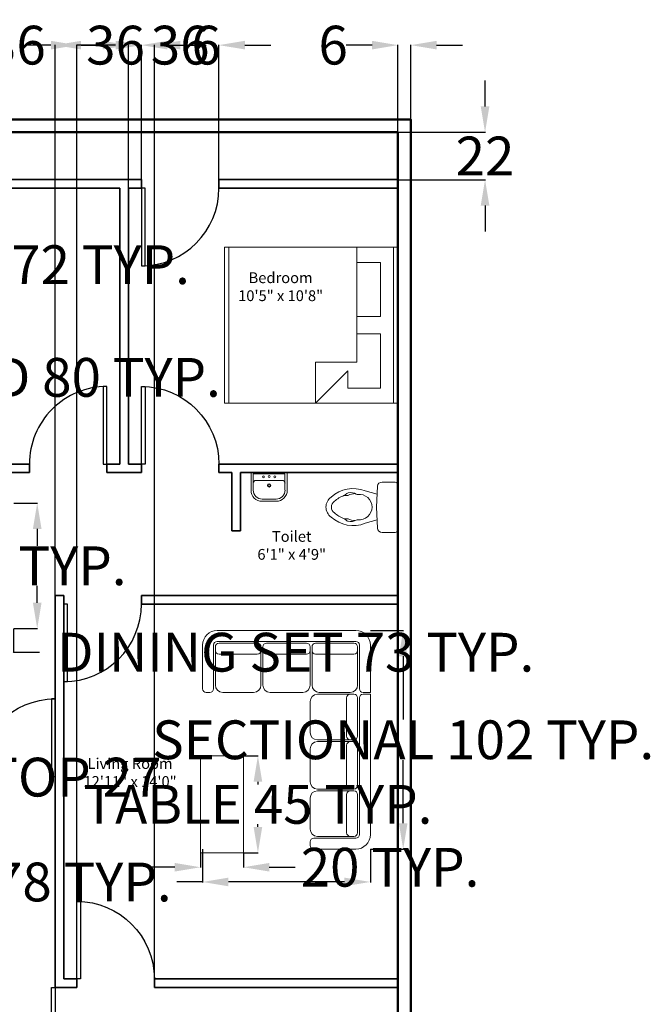
# Model space of a CAD drawing. Units: inches. Extents: x -230 to 384, y -962 to -183.
# Tile 6 of 6: x 91 to 384, y -640 to -183. Entities that reach past the tile are written whole.
import ezdxf

# ---------------------------------------------------------------- set-up
doc = ezdxf.new("R2010")
doc.units = ezdxf.units.IN
for name, color, linetype, lineweight in [('A-ANNO-DIMS', 2, 'Continuous', 18), ('A-AREA-IDEN', 7, 'Continuous', 18), ('A-DOOR', 3, 'Continuous', 25), ('A-FLOR-FIXT', 9, 'Continuous', 18), ('Furniture', 2, 'Continuous', 18), ('Inner Wall', 5, 'Continuous', 35), ('Outer Wall', 1, 'Continuous', 50)]:
    doc.layers.add(name, color=color, linetype=linetype, lineweight=lineweight)
doc.styles.get("Standard").update_dxf_attribs({"font": 'arial.ttf'})
doc.dimstyles.get("Standard").update_dxf_attribs({"dimtxt": 18, "dimasz": 12, "dimexe": 0.18, "dimexo": 0.0625, "dimgap": 0.09, "dimtad": 0, "dimtih": 1, "dimtoh": 1, "dimdec": 0, "dimzin": 0, "dimdsep": 46, "dimlunit": 3, "dimtxsty": 'Standard', "dimcen": 0.09, "dimadec": 0, "dimazin": 0, "dimtfac": 1, "dimtdec": 0, "dimtofl": 0, "dimtmove": 0, "dimatfit": 3, "dimfxl": 1, "dimtolj": 1, "dimtzin": 0, "dimarcsym": 0})

# ---------------------------------------------------------------- blocks, each defined once
blk = doc.blocks.new('*U2')
for p, q in [((0, 0), (0, 4)), ((36, 0), (36, 4))]:
    blk.add_line(p, q)
blk.add_lwpolyline([(0, 0), (0, -36), (1.75, -36), (1.75, 0)], close=True)
blk.add_arc((0, 0), 36, 270, 0)
blk = doc.blocks.new('*U4')
for p, q in [((0, 0), (0, -4)), ((36, 0), (36, -4))]:
    blk.add_line(p, q)
blk.add_lwpolyline([(0, 0), (0, 36), (1.75, 36), (1.75, 0)], close=True)
blk.add_arc((0, 0), 36, 0, 90)
blk = doc.blocks.new('A$C2AFA021D')
for p, q in [((0.8, 2.3), (0.2, 2.3)), ((0.85, 2.2), (0.85, 2.25)), ((0, 2.1), (0, 0.2)), ((0.15, 0.2), (0.15, 2.1)), ((0.175, 1.55), (0.175, 2.075)), ((0.2, 2.15), (0.8, 2.15)), ((0.225, 2.125), (0.275, 2.125)), ((0.75, 2.125), (0.275, 2.125)), ((0.325, 2.075), (0.325, 1.55)), ((0.85, 1.6), (0.85, 2.025)), ((0.275, 1.5), (0.225, 1.5)), ((0.275, 1.5), (0.75, 1.5)), ((0.175, 0.875), (0.175, 1.425)), ((0.225, 1.475), (0.275, 1.475)), ((0.75, 1.475), (0.275, 1.475)), ((0.325, 1.425), (0.325, 0.875)), ((0.85, 0.925), (0.85, 1.375)), ((0.275, 0.825), (0.225, 0.825)), ((0.275, 0.825), (0.75, 0.825)), ((0.975, 0.825), (1.4, 0.825)), ((1.625, 0.825), (2.075, 0.825)), ((2.3, 0.825), (2.725, 0.825)), ((2.9, 0.825), (2.95, 0.825)), ((0.175, 0.225), (0.175, 0.75)), ((0.225, 0.8), (0.275, 0.8)), ((0.75, 0.8), (0.275, 0.8)), ((0.325, 0.75), (0.325, 0.225)), ((0.85, 0.275), (0.85, 0.7)), ((0.875, 0.275), (0.875, 0.725)), ((1.5, 0.725), (1.5, 0.275)), ((1.525, 0.275), (1.525, 0.725)), ((2.175, 0.725), (2.175, 0.275)), ((2.2, 0.275), (2.2, 0.725)), ((2.825, 0.725), (2.825, 0.275)), ((2.85, 0.2), (2.85, 0.775)), ((3, 0.775), (3, 0.2)), ((0.875, 0.275), (0.875, 0.225)), ((1.45, 0.325), (0.925, 0.325)), ((1.5, 0.225), (1.5, 0.275)), ((1.525, 0.275), (1.525, 0.225)), ((2.125, 0.325), (1.575, 0.325)), ((2.175, 0.225), (2.175, 0.275)), ((2.2, 0.275), (2.2, 0.225)), ((2.775, 0.325), (2.25, 0.325)), ((2.825, 0.225), (2.825, 0.275)), ((0.8, 0.15), (0.2, 0.15)), ((0.275, 0.175), (0.225, 0.175)), ((0.275, 0.175), (0.75, 0.175)), ((0.925, 0.175), (1.45, 0.175)), ((0.925, 0.15), (2.8, 0.15)), ((1.575, 0.175), (2.125, 0.175)), ((2.25, 0.175), (2.775, 0.175)), ((0.85, 0), (0.85, 0.1)), ((0.875, 0.1), (0.875, 0)), ((0.2, 0), (0.85, 0)), ((2.8, 0), (0.875, 0))]:
    blk.add_line(p, q)
for centre, radius, start, end in [((0.2, 2.1), 0.2, 90, 180), ((0.8, 2.25), 0.05, 0, 90), ((0.8, 2.2), 0.05, 270, 0), ((0.2, 2.1), 0.05, 90, 180), ((0.225, 2.075), 0.05, 90, 180), ((0.275, 2.075), 0.05, 0, 90), ((0.75, 2.025), 0.1, 0, 90), ((0.225, 1.55), 0.05, 180, 270), ((0.275, 1.55), 0.05, 270, 0), ((0.75, 1.6), 0.1, 270, 0), ((0.225, 1.425), 0.05, 90, 180), ((0.275, 1.425), 0.05, 0, 90), ((0.75, 1.375), 0.1, 360, 90), ((0.225, 0.875), 0.05, 180, 270), ((0.275, 0.875), 0.05, 270, 0), ((0.75, 0.925), 0.1, 270, 0), ((0.975, 0.725), 0.1, 90, 180), ((1.4, 0.725), 0.1, 0, 90), ((1.625, 0.725), 0.1, 90, 180), ((2.075, 0.725), 0.1, 0, 90), ((2.3, 0.725), 0.1, 90, 180), ((2.725, 0.725), 0.1, 0, 90), ((2.9, 0.775), 0.05, 90, 180), ((2.95, 0.775), 0.05, 0, 90), ((0.225, 0.75), 0.05, 90, 180), ((0.275, 0.75), 0.05, 0, 90), ((0.75, 0.7), 0.1, 0, 90), ((0.75, 0.275), 0.1, 270, 0), ((0.925, 0.275), 0.05, 90, 180), ((1.45, 0.275), 0.05, 360, 90), ((1.575, 0.275), 0.05, 90, 180), ((2.125, 0.275), 0.05, 360, 90), ((2.25, 0.275), 0.05, 90, 180), ((2.775, 0.275), 0.05, 360, 90), ((0.2, 0.2), 0.2, 180, 270), ((0.2, 0.2), 0.05, 180, 270), ((0.225, 0.225), 0.05, 180, 270), ((0.275, 0.225), 0.05, 270, 0), ((0.8, 0.1), 0.05, 0, 90), ((0.925, 0.225), 0.05, 180, 270), ((0.925, 0.1), 0.05, 90, 180), ((1.45, 0.225), 0.05, 270, 0), ((1.575, 0.225), 0.05, 180, 270), ((2.125, 0.225), 0.05, 270, 0), ((2.25, 0.225), 0.05, 180, 270), ((2.775, 0.225), 0.05, 270, 0), ((2.8, 0.2), 0.2, 270, 0), ((2.8, 0.2), 0.05, 270, 0)]:
    blk.add_arc(centre, radius, start, end)
blk = doc.blocks.new('KING-00')
for p, q in [((-0.897, -0.947), (-0.897, 0.882)), ((0.602, 0.882), (0.602, -0.464)), ((1.034, -0.947), (1.034, 0.882)), ((0.602, 0.704), (0.881, 0.704)), ((0.881, 0.069), (0.881, 0.704)), ((0.602, 0.069), (0.881, 0.069)), ((0.881, -0.134), (0.602, -0.134)), ((0.881, -0.769), (0.881, -0.134)), ((0.119, -0.464), (0.119, -0.947)), ((0.602, -0.464), (0.119, -0.464)), ((0.119, -0.947), (0.5, -0.566)), ((0.5, -0.769), (0.5, -0.566)), ((0.5, -0.769), (0.881, -0.769))]:
    blk.add_line(p, q)
blk.add_lwpolyline([(-0.948, -0.947), (-0.948, 0.882), (1.084, 0.882), (1.084, -0.947)], close=True)
blk = doc.blocks.new('A$C1308471B')
at = {"ltscale": 20}
for p, q in [((0.0354, 0.4793), (0.1495, 0.4793)), ((0, 0.4607), (0, 0.0186)), ((0.2013, 0.2397), (0.1923, 0.4384)), ((0.1957, 0.3639), (0.3109, 0.3953)), ((0.5021, 0.3528), (0.4724, 0.3528)), ((0.4982, 0.3575), (0.4822, 0.3709)), ((0.2013, 0.2397), (0.1923, 0.0409)), ((0.1959, 0.1193), (0.3109, 0.0879)), ((0.5021, 0.1304), (0.4724, 0.1304)), ((0.4982, 0.1257), (0.4822, 0.1123)), ((0.0354, 0), (0.1495, 0))]:
    blk.add_line(p, q, dxfattribs=at)
for centre, radius, start, end in [((0.0354, 0.4328), 0.0465, 90, 136.52689), ((0.1495, 0.4365), 0.0429, 2.57554, 90), ((0.006, 0.4607), 0.006, 136.52689, 180), ((0.4248, 0.1104), 0.3068, 47.41345, 111.79241), ((0.4494, 0.2636), 0.1148, 79.39683, 118.57415), ((0.4658, 0.3513), 0.0255, 50, 79.39683), ((0.3654, 0.2416), 0.1206, 83.35226, 180), ((0.3823, 0.3868), 0.0255, 263.35226, 298.57415), ((0.405, 0.2159), 0.153, 63.50202, 90.45216), ((0.5146, 0.377), 0.0255, 230, 251.38812), ((0.5021, 0.3273), 0.0255, 70.3751, 90), ((0.4248, 0.1104), 0.2558, 46.61198, 70.3751), ((0.5654, 0.2416), 0.065, 0, 57.29738), ((0.5654, 0.2416), 0.116, 0, 54.71147), ((0.3654, 0.2416), 0.1206, 180, 276.64774), ((0.4248, 0.3728), 0.2558, 289.6249, 313.38802), ((0.5654, 0.2416), 0.065, 302.70262, 0), ((0.5654, 0.2416), 0.116, 305.28853, 0), ((0.4248, 0.3728), 0.3068, 248.20759, 312.58655), ((0.3823, 0.0964), 0.0255, 61.42585, 96.64774), ((0.4494, 0.2196), 0.1148, 241.42585, 280.60317), ((0.405, 0.2673), 0.153, 269.54784, 296.49798), ((0.4658, 0.1319), 0.0255, 280.60317, 310), ((0.5146, 0.1062), 0.0255, 108.61188, 130), ((0.5021, 0.1559), 0.0255, 270, 289.6249), ((0.006, 0.0186), 0.006, 180, 223.47311), ((0.0354, 0.0465), 0.0465, 223.47311, 270), ((0.1495, 0.0429), 0.0429, 270, 357.42446)]:
    blk.add_arc(centre, radius, start, end, dxfattribs=at)
blk = doc.blocks.new('A$C57EA129C')
for p, q in [((0, 0.443), (0, 0.178)), ((0.016, 0.459), (0.563, 0.459)), ((0.036, 0.432), (0.036, 0.29)), ((0.045, 0.441), (0.535, 0.441)), ((0.08, 0.334), (0.499, 0.334)), ((0.544, 0.432), (0.544, 0.29)), ((0.579, 0.443), (0.579, 0.178)), ((0.036, 0.29), (0.036, 0.178)), ((0.544, 0.29), (0.544, 0.178)), ((0.178, 0.036), (0.401, 0.036)), ((0.178, 0), (0.401, 0))]:
    blk.add_line(p, q)
for centre, radius in [((0.198, 0.392), 0.0143), ((0.29, 0.396), 0.0156), ((0.381, 0.392), 0.0143), ((0.29, 0.255), 0.0267), ((0.29, 0.255), 0.0178)]:
    blk.add_circle(centre, radius)
for centre, radius, start, end in [((0.016, 0.443), 0.016, 90, 180), ((0.045, 0.432), 0.00891, 90, 180), ((0.08, 0.29), 0.0445, 90, 180), ((0.499, 0.29), 0.0445, 0, 90), ((0.535, 0.432), 0.00891, 0, 90), ((0.563, 0.443), 0.016, 0, 90), ((0.178, 0.178), 0.178, 180, 270), ((0.178, 0.178), 0.143, 180, 270), ((0.401, 0.178), 0.178, 270, 0), ((0.401, 0.178), 0.143, 270, 0)]:
    blk.add_arc(centre, radius, start, end)
blk = doc.blocks.new('TABLE-COFFEE-RECT')
blk.add_lwpolyline([(0, 44.94), (19.86, 44.94), (19.86, 0), (0, 0)], close=True)
blk = doc.blocks.new('*D16')
at = {"layer": 'A-ANNO-DIMS', "color": 0, "lineweight": -2, "transparency": 16777216}
for p, q in [((72.67, -308.78), (84.86, -308.78)), ((84.68, -320.78), (84.68, -339.62)), ((84.68, -377.25), (84.68, -358.42)), ((72.67, -389.25), (84.86, -389.25))]:
    blk.add_line(p, q, dxfattribs=at)
at = {"layer": 'A-ANNO-DIMS', "color": 0, "transparency": 16777216}
for points in [[(82.68, -320.78), (86.68, -320.78), (84.68, -308.78)], [(82.68, -377.25), (86.68, -377.25), (84.68, -389.25)]]:
    blk.add_solid(points, dxfattribs=at)
at = {"layer": 'Defpoints', "color": 0, "transparency": 16777216}
for p in [(72.61, -308.78), (72.61, -389.25), (84.68, -389.25)]:
    blk.add_point(p, dxfattribs=at)
at = {"layer": 'A-ANNO-DIMS', "color": 0, "transparency": 16777216, "insert": (84.68, -349.02), "char_height": 18, "attachment_point": 5}
blk.add_mtext('\\A1;KING BED 80 TYP.', dxfattribs=at)
blk = doc.blocks.new('*D17')
at = {"layer": 'A-ANNO-DIMS', "color": 0, "lineweight": -2, "transparency": 16777216}
for p, q in [((0.19, -308.72), (0.19, -296.53)), ((12.19, -296.71), (60.61, -296.71)), ((72.61, -308.72), (72.61, -296.53)), ((72.61, -296.71), (84.61, -296.71))]:
    blk.add_line(p, q, dxfattribs=at)
at = {"layer": 'A-ANNO-DIMS', "color": 0, "transparency": 16777216}
for points in [[(12.19, -294.71), (12.19, -298.71), (0.19, -296.71)], [(60.61, -294.71), (60.61, -298.71), (72.61, -296.71)]]:
    blk.add_solid(points, dxfattribs=at)
at = {"layer": 'Defpoints', "color": 0, "transparency": 16777216}
for p in [(72.61, -296.71), (0.19, -308.78), (72.61, -308.78)]:
    blk.add_point(p, dxfattribs=at)
at = {"layer": 'A-ANNO-DIMS', "color": 0, "transparency": 16777216, "insert": (128.44, -296.71), "char_height": 18, "attachment_point": 5}
blk.add_mtext('\\A1;72 TYP.', dxfattribs=at)
blk = doc.blocks.new('*D22')
at = {"layer": 'A-ANNO-DIMS', "color": 0, "lineweight": -2, "transparency": 16777216}
for p, q in [((253.7, -466.5), (269.04, -466.5)), ((268.86, -478.5), (268.86, -507.86)), ((268.86, -556.02), (268.86, -526.67)), ((253.7, -568.02), (269.04, -568.02))]:
    blk.add_line(p, q, dxfattribs=at)
at = {"layer": 'A-ANNO-DIMS', "color": 0, "transparency": 16777216}
for points in [[(266.86, -478.5), (270.86, -478.5), (268.86, -466.5)], [(266.86, -556.02), (270.86, -556.02), (268.86, -568.02)]]:
    blk.add_solid(points, dxfattribs=at)
at = {"layer": 'Defpoints', "color": 0, "transparency": 16777216}
for p in [(253.63, -466.5), (253.63, -568.02), (268.86, -568.02)]:
    blk.add_point(p, dxfattribs=at)
at = {"layer": 'A-ANNO-DIMS', "color": 0, "transparency": 16777216, "insert": (268.86, -517.26), "char_height": 18, "attachment_point": 5}
blk.add_mtext('\\A1;SECTIONAL 102 TYP.', dxfattribs=at)
blk = doc.blocks.new('*D23')
at = {"layer": 'A-ANNO-DIMS', "color": 0, "lineweight": -2, "transparency": 16777216}
for p, q in [((175.8, -568.08), (175.8, -583.43)), ((253.63, -568.08), (253.63, -583.43)), ((175.8, -583.25), (163.8, -583.25)), ((241.63, -583.25), (187.8, -583.25))]:
    blk.add_line(p, q, dxfattribs=at)
at = {"layer": 'A-ANNO-DIMS', "color": 0, "transparency": 16777216}
for points in [[(187.8, -581.25), (187.8, -585.25), (175.8, -583.25)], [(241.63, -581.25), (241.63, -585.25), (253.63, -583.25)]]:
    blk.add_solid(points, dxfattribs=at)
at = {"layer": 'Defpoints', "color": 0, "transparency": 16777216}
for p in [(175.8, -568.02), (253.63, -568.02), (175.8, -583.25)]:
    blk.add_point(p, dxfattribs=at)
at = {"layer": 'A-ANNO-DIMS', "color": 0, "transparency": 16777216, "insert": (119.97, -583.25), "char_height": 18, "attachment_point": 5}
blk.add_mtext('\\A1;78 TYP.', dxfattribs=at)
blk = doc.blocks.new('*D24')
at = {"layer": 'A-ANNO-DIMS', "color": 0, "lineweight": -2, "transparency": 16777216}
for p, q in [((14.93, -465.69), (14.93, -476.78)), ((88.09, -465.69), (88.09, -476.78)), ((26.93, -476.6), (76.09, -476.6)), ((88.09, -476.6), (100.09, -476.6))]:
    blk.add_line(p, q, dxfattribs=at)
at = {"layer": 'A-ANNO-DIMS', "color": 0, "transparency": 16777216}
for points in [[(26.93, -474.6), (26.93, -478.6), (14.93, -476.6)], [(76.09, -474.6), (76.09, -478.6), (88.09, -476.6)]]:
    blk.add_solid(points, dxfattribs=at)
at = {"layer": 'Defpoints', "color": 0, "transparency": 16777216}
for p in [(14.93, -465.63), (88.09, -465.63), (88.09, -476.6)]:
    blk.add_point(p, dxfattribs=at)
at = {"layer": 'A-ANNO-DIMS', "color": 0, "transparency": 16777216, "insert": (218.98, -476.6), "char_height": 18, "attachment_point": 5}
blk.add_mtext('\\A1;DINING SET 73 TYP.', dxfattribs=at)
blk = doc.blocks.new('*D25')
at = {"layer": 'A-ANNO-DIMS', "color": 0, "lineweight": -2, "transparency": 16777216}
for p, q in [((88.15, -407.34), (99.24, -407.34)), ((99.06, -419.34), (99.06, -427.2)), ((99.06, -453.63), (99.06, -445.76)), ((88.15, -465.63), (99.24, -465.63))]:
    blk.add_line(p, q, dxfattribs=at)
at = {"layer": 'A-ANNO-DIMS', "color": 0, "transparency": 16777216}
for points in [[(97.06, -419.34), (101.06, -419.34), (99.06, -407.34)], [(97.06, -453.63), (101.06, -453.63), (99.06, -465.63)]]:
    blk.add_solid(points, dxfattribs=at)
at = {"layer": 'Defpoints', "color": 0, "transparency": 16777216}
for p in [(88.09, -407.34), (99.06, -407.34), (88.09, -465.63)]:
    blk.add_point(p, dxfattribs=at)
at = {"layer": 'A-ANNO-DIMS', "color": 0, "transparency": 16777216, "insert": (99.06, -436.48), "char_height": 18, "attachment_point": 5}
blk.add_mtext('\\A1;58 TYP.', dxfattribs=at)
blk = doc.blocks.new('*D26')
at = {"layer": 'A-ANNO-DIMS', "color": 0, "lineweight": -2, "transparency": 16777216}
for p, q in [((194.78, -524.74), (201.64, -524.74)), ((201.46, -536.74), (201.46, -537.96)), ((201.46, -557.68), (201.46, -556.45)), ((194.78, -569.68), (201.64, -569.68))]:
    blk.add_line(p, q, dxfattribs=at)
at = {"layer": 'A-ANNO-DIMS', "color": 0, "transparency": 16777216}
for points in [[(199.46, -536.74), (203.46, -536.74), (201.46, -524.74)], [(199.46, -557.68), (203.46, -557.68), (201.46, -569.68)]]:
    blk.add_solid(points, dxfattribs=at)
at = {"layer": 'Defpoints', "color": 0, "transparency": 16777216}
for p in [(194.72, -524.74), (201.46, -524.74), (194.72, -569.68)]:
    blk.add_point(p, dxfattribs=at)
at = {"layer": 'A-ANNO-DIMS', "color": 0, "transparency": 16777216, "insert": (201.46, -547.21), "char_height": 18, "attachment_point": 5}
blk.add_mtext('\\A1;TABLE 45 TYP.', dxfattribs=at)
blk = doc.blocks.new('*D27')
at = {"layer": 'A-ANNO-DIMS', "color": 0, "lineweight": -2, "transparency": 16777216}
for p, q in [((174.85, -569.74), (174.85, -576.6)), ((194.72, -569.74), (194.72, -576.6)), ((162.85, -576.42), (150.85, -576.42)), ((206.72, -576.42), (218.72, -576.42))]:
    blk.add_line(p, q, dxfattribs=at)
at = {"layer": 'A-ANNO-DIMS', "color": 0, "transparency": 16777216}
for points in [[(162.85, -574.42), (162.85, -578.42), (174.85, -576.42)], [(206.72, -574.42), (206.72, -578.42), (194.72, -576.42)]]:
    blk.add_solid(points, dxfattribs=at)
at = {"layer": 'Defpoints', "color": 0, "transparency": 16777216}
for p in [(174.85, -569.68), (194.72, -569.68), (194.72, -576.42)]:
    blk.add_point(p, dxfattribs=at)
at = {"layer": 'A-ANNO-DIMS', "color": 0, "transparency": 16777216, "insert": (262.77, -576.42), "char_height": 18, "attachment_point": 5}
blk.add_mtext('\\A1;20 TYP.', dxfattribs=at)
blk = doc.blocks.new('*D28')
at = {"layer": 'A-ANNO-DIMS', "color": 0, "lineweight": -2, "transparency": 16777216}
for p, q in [((-36.67, -530.52), (-36.67, -534.76)), ((-24.67, -534.58), (-21.19, -534.58)), ((-9.19, -530.52), (-9.19, -534.76)), ((-9.19, -534.58), (2.81, -534.58))]:
    blk.add_line(p, q, dxfattribs=at)
at = {"layer": 'A-ANNO-DIMS', "color": 0, "transparency": 16777216}
for points in [[(-24.67, -532.58), (-24.67, -536.58), (-36.67, -534.58)], [(-21.19, -532.58), (-21.19, -536.58), (-9.19, -534.58)]]:
    blk.add_solid(points, dxfattribs=at)
at = {"layer": 'Defpoints', "color": 0, "transparency": 16777216}
for p in [(-36.67, -530.46), (-9.19, -530.46), (-9.19, -534.58)]:
    blk.add_point(p, dxfattribs=at)
at = {"layer": 'A-ANNO-DIMS', "color": 0, "transparency": 16777216, "insert": (82.05, -534.58), "char_height": 18, "attachment_point": 5}
blk.add_mtext('\\A1;COOKTOP 27', dxfattribs=at)
blk = doc.blocks.new('*D34')
at = {"layer": 'A-ANNO-DIMS', "color": 0, "lineweight": -2, "transparency": 16777216}
for p, q in [((306.84801, -223.25445), (306.84801, -211.25445)), ((266.46051, -235.25445), (307.02801, -235.25445)), ((266.46051, -257.25445), (307.02801, -257.25445)), ((306.84801, -269.25445), (306.84801, -281.25445))]:
    blk.add_line(p, q, dxfattribs=at)
at = {"layer": 'A-ANNO-DIMS', "color": 0, "transparency": 16777216}
for points in [[(304.84801, -223.25445), (308.84801, -223.25445), (306.84801, -235.25445)], [(304.84801, -269.25445), (308.84801, -269.25445), (306.84801, -257.25445)]]:
    blk.add_solid(points, dxfattribs=at)
at = {"layer": 'Defpoints', "color": 0, "transparency": 16777216}
for p in [(266.39801, -235.25445), (266.39801, -257.25445), (306.84801, -257.25445)]:
    blk.add_point(p, dxfattribs=at)
at = {"layer": 'A-ANNO-DIMS', "color": 0, "transparency": 16777216, "insert": (306.84801, -246.25445), "char_height": 18, "attachment_point": 5}
blk.add_mtext('\\A1;22', dxfattribs=at)
blk = doc.blocks.new('*D37')
at = {"layer": 'A-ANNO-DIMS', "color": 0, "lineweight": -2, "transparency": 16777216}
for p, q in [((135.39801, -194.80445), (123.39801, -194.80445)), ((147.39801, -257.19195), (147.39801, -194.62445)), ((183.39801, -257.19195), (183.39801, -194.62445)), ((195.39801, -194.80445), (207.39801, -194.80445))]:
    blk.add_line(p, q, dxfattribs=at)
at = {"layer": 'A-ANNO-DIMS', "color": 0, "transparency": 16777216}
for points in [[(135.39801, -192.80445), (135.39801, -196.80445), (147.39801, -194.80445)], [(195.39801, -192.80445), (195.39801, -196.80445), (183.39801, -194.80445)]]:
    blk.add_solid(points, dxfattribs=at)
at = {"layer": 'Defpoints', "color": 0, "transparency": 16777216}
for p in [(183.39801, -194.80445), (147.39801, -257.25445), (183.39801, -257.25445)]:
    blk.add_point(p, dxfattribs=at)
at = {"layer": 'A-ANNO-DIMS', "color": 0, "transparency": 16777216, "insert": (165.39801, -194.80445), "char_height": 18, "attachment_point": 5}
blk.add_mtext('\\A1;36', dxfattribs=at)
blk = doc.blocks.new('*D44')
at = {"layer": 'A-ANNO-DIMS', "color": 0, "lineweight": -2, "transparency": 16777216}
for p, q in [((254.4, -194.8), (242.4, -194.8)), ((266.4, -235.19), (266.4, -194.62)), ((272.4, -229.19), (272.4, -194.62)), ((284.4, -194.8), (296.4, -194.8))]:
    blk.add_line(p, q, dxfattribs=at)
at = {"layer": 'A-ANNO-DIMS', "color": 0, "transparency": 16777216}
for points in [[(254.4, -192.8), (254.4, -196.8), (266.4, -194.8)], [(284.4, -192.8), (284.4, -196.8), (272.4, -194.8)]]:
    blk.add_solid(points, dxfattribs=at)
at = {"layer": 'Defpoints', "color": 0, "transparency": 16777216}
for p in [(266.4, -194.8), (272.4, -229.25), (266.4, -235.25)]:
    blk.add_point(p, dxfattribs=at)
at = {"layer": 'A-ANNO-DIMS', "color": 0, "transparency": 16777216, "insert": (236.37, -194.8), "char_height": 18, "attachment_point": 5}
blk.add_mtext('\\A1;6', dxfattribs=at)
blk = doc.blocks.new('*D49')
at = {"layer": 'A-ANNO-DIMS', "color": 0, "lineweight": -2, "transparency": 16777216}
for p, q in [((129.4, -194.8), (117.4, -194.8)), ((141.4, -261.19), (141.4, -194.62)), ((147.4, -257.19), (147.4, -194.62)), ((159.4, -194.8), (171.4, -194.8))]:
    blk.add_line(p, q, dxfattribs=at)
at = {"layer": 'A-ANNO-DIMS', "color": 0, "transparency": 16777216}
for points in [[(129.4, -192.8), (129.4, -196.8), (141.4, -194.8)], [(159.4, -192.8), (159.4, -196.8), (147.4, -194.8)]]:
    blk.add_solid(points, dxfattribs=at)
at = {"layer": 'Defpoints', "color": 0, "transparency": 16777216}
for p in [(147.4, -194.8), (147.4, -257.25), (141.4, -261.25)]:
    blk.add_point(p, dxfattribs=at)
at = {"layer": 'A-ANNO-DIMS', "color": 0, "transparency": 16777216, "insert": (177.43, -194.8), "char_height": 18, "attachment_point": 5}
blk.add_mtext('\\A1;6', dxfattribs=at)
blk = doc.blocks.new('*D50')
at = {"layer": 'A-ANNO-DIMS', "color": 0, "lineweight": -2, "transparency": 16777216}
for p, q in [((59.39801, -194.80445), (47.39801, -194.80445)), ((71.39801, -534.19195), (71.39801, -194.62445)), ((107.39801, -534.19195), (107.39801, -194.62445)), ((119.39801, -194.80445), (131.39801, -194.80445))]:
    blk.add_line(p, q, dxfattribs=at)
at = {"layer": 'A-ANNO-DIMS', "color": 0, "transparency": 16777216}
for points in [[(59.39801, -192.80445), (59.39801, -196.80445), (71.39801, -194.80445)], [(119.39801, -192.80445), (119.39801, -196.80445), (107.39801, -194.80445)]]:
    blk.add_solid(points, dxfattribs=at)
at = {"layer": 'Defpoints', "color": 0, "transparency": 16777216}
for p in [(107.39801, -194.80445), (71.39801, -534.25445), (107.39801, -534.25445)]:
    blk.add_point(p, dxfattribs=at)
at = {"layer": 'A-ANNO-DIMS', "color": 0, "transparency": 16777216, "insert": (89.39801, -194.80445), "char_height": 18, "attachment_point": 5}
blk.add_mtext('\\A1;36', dxfattribs=at)
blk = doc.blocks.new('*D52')
at = {"layer": 'A-ANNO-DIMS', "color": 0, "lineweight": -2, "transparency": 16777216}
for p, q in [((105.39801, -194.80445), (93.39801, -194.80445)), ((117.39801, -628.19195), (117.39801, -194.62445)), ((153.39801, -628.19195), (153.39801, -194.62445)), ((165.39801, -194.80445), (177.39801, -194.80445))]:
    blk.add_line(p, q, dxfattribs=at)
at = {"layer": 'A-ANNO-DIMS', "color": 0, "transparency": 16777216}
for points in [[(105.39801, -192.80445), (105.39801, -196.80445), (117.39801, -194.80445)], [(165.39801, -192.80445), (165.39801, -196.80445), (153.39801, -194.80445)]]:
    blk.add_solid(points, dxfattribs=at)
at = {"layer": 'Defpoints', "color": 0, "transparency": 16777216}
for p in [(153.39801, -194.80445), (117.39801, -628.25445), (153.39801, -628.25445)]:
    blk.add_point(p, dxfattribs=at)
at = {"layer": 'A-ANNO-DIMS', "color": 0, "transparency": 16777216, "insert": (135.39801, -194.80445), "char_height": 18, "attachment_point": 5}
blk.add_mtext('\\A1;36', dxfattribs=at)

msp = doc.modelspace()

# ---------------------------------------------------------------- linework, layer by layer
at = {"layer": 'Inner Wall'}
for p, q in [((-41.6, -257.25), (147.4, -257.25)), ((147.4, -257.25), (147.4, -261.25)), ((183.4, -257.25), (183.4, -261.25)), ((183.4, -257.25), (266.4, -257.25)), ((-41.6, -261.25), (137.4, -261.25)), ((137.4, -261.25), (137.4, -389.25)), ((141.4, -261.25), (141.4, -389.25)), ((141.4, -261.25), (147.4, -261.25)), ((183.4, -261.25), (266.4, -261.25)), ((-22.6, -389.25), (95.4, -389.25)), ((95.4, -389.25), (95.4, -393.25)), ((131.4, -389.25), (131.4, -393.25)), ((131.4, -389.25), (137.4, -389.25)), ((141.4, -389.25), (147.4, -389.25)), ((147.4, -389.25), (147.4, -393.25)), ((183.4, -389.25), (183.4, -393.25)), ((183.4, -389.25), (266.4, -389.25)), ((-18.6, -393.25), (95.4, -393.25)), ((131.4, -393.25), (147.4, -393.25)), ((183.4, -393.25), (189.4, -393.25)), ((189.4, -393.25), (189.4, -420.25)), ((193.4, -393.25), (193.4, -420.25)), ((193.4, -393.25), (266.4, -393.25)), ((189.4, -420.25), (193.4, -420.25)), ((107.4, -450.25), (111.4, -450.25)), ((107.4, -450.25), (107.4, -632.25)), ((111.4, -450.25), (111.4, -628.25)), ((147.4, -450.25), (147.4, -454.25)), ((147.4, -450.25), (266.4, -450.25)), ((147.4, -454.25), (266.4, -454.25)), ((111.4, -628.25), (117.4, -628.25)), ((117.4, -628.25), (117.4, -632.25)), ((153.4, -628.25), (153.4, -632.25)), ((153.4, -628.25), (266.4, -628.25)), ((107.4, -632.25), (117.4, -632.25)), ((153.4, -632.25), (266.4, -632.25))]:
    msp.add_line(p, q, dxfattribs=at)
at = {"layer": 'Outer Wall'}
for p, q in [((-95.6, -235.25), (266.4, -235.25)), ((266.4, -235.25), (266.4, -909.25))]:
    msp.add_line(p, q, dxfattribs=at)
msp.add_lwpolyline([(272.4, -915.25), (-101.6, -915.25), (-101.6, -229.25), (272.4, -229.25)], close=True, dxfattribs=at)

# ---------------------------------------------------------------- block references
at = {"layer": 'A-DOOR'}
for p in [(147.4, -261.25), (111.4, -454.25)]:
    msp.add_blockref('*U2', p, dxfattribs=at)
at = {"layer": 'A-DOOR', "rotation": 180}
for name, p in [('*U2', (131.4, -389.25)), ('*U4', (107.4, -632.25))]:
    msp.add_blockref(name, p, dxfattribs=at)
at = {"layer": 'A-DOOR', "xscale": -1, "rotation": 180}
for p in [(147.4, -389.25), (117.4, -628.25)]:
    msp.add_blockref('*U2', p, dxfattribs=at)
at = {"layer": 'A-DOOR', "xscale": -1}
msp.add_blockref('*U4', (107.4, -534.25), dxfattribs=at)
at = {"layer": 'A-FLOR-FIXT'}
for name, p, xscale, yscale, zscale in [('A$C57EA129C', (215.06, -406.55), -28.98333223671166, 28.98333223671166, 28.98333223671166), ('A$C1308471B', (266.4, -421.06), -48.95497407897215, 48.95497407897215, 48.95497407897215)]:
    msp.add_blockref(name, p, dxfattribs=dict(at, xscale=xscale, yscale=yscale, zscale=zscale))
at = {"layer": 'Furniture', "xscale": 39.60249106241186, "yscale": 39.60249106241186, "zscale": 39.60249106241186}
msp.add_blockref('KING-00', (223.45, -323.56), dxfattribs=at)
at = {"layer": 'Furniture', "xscale": -33.84012530478223, "yscale": 33.84012530478223, "zscale": 33.84012530478223, "rotation": 90}
msp.add_blockref('A$C2AFA021D', (253.63, -466.5), dxfattribs=at)
at = {"layer": 'Furniture'}
msp.add_blockref('TABLE-COFFEE-RECT', (174.85, -569.68), dxfattribs=at)

# ---------------------------------------------------------------- texts
at = {"layer": 'A-AREA-IDEN', "char_height": 5, "attachment_point": 3}
for s, insert in [('\\pxqc;{\\fTimes New Roman|b0|i0|c0|p18;Bedroom\\P10\'5" x 10\'8"}', (236.55, -300.28)), ('\\pxqc;{\\fTimes New Roman|b0|i0|c0|p18;Toilet\\P6\'1" x 4\'9"}', (241.69, -420.35)), ('\\pxqc;{\\fTimes New Roman|b0|i0|c0|p18;Living Room\\P12\'11" x 14\'0"}', (166.68, -525.78))]:
    msp.add_mtext_dynamic_manual_height_columns(s, width=49.1019, gutter_width=12.5, heights=[0], dxfattribs=dict(at, insert=insert))

# ---------------------------------------------------------------- dimensions: what is measured, and where the dimension line sits
at = {"layer": 'A-ANNO-DIMS'}
for base, p1, p2, picture, middle in [((107.4, -194.8), (71.4, -534.25), (107.4, -534.25), '*D50', (89.4, -194.8)), ((153.4, -194.8), (117.4, -628.25), (153.4, -628.25), '*D52', (135.4, -194.8)), ((147.4, -194.8), (141.4, -261.25), (147.4, -257.25), '*D49', (177.43, -194.8)), ((183.4, -194.8), (147.4, -257.25), (183.4, -257.25), '*D37', (165.4, -194.8)), ((266.4, -194.8), (272.4, -229.25), (266.4, -235.25), '*D44', (236.37, -194.8))]:
    dim = msp.add_linear_dim(base=base, p1=p1, p2=p2, dimstyle='Standard', override={"dimdec": 0, "dimlfac": 1, "dimrnd": 0, "dimzin": 0, "dimdsep": 46, "dimlunit": 2}, dxfattribs=at)
    dim.commit()
    dim.dimension.update_dxf_attribs({"geometry": picture, "text_midpoint": middle})
dim = msp.add_linear_dim(base=(306.85, -257.25), p1=(266.4, -235.25), p2=(266.4, -257.25), angle=90, dimstyle='Standard', override={"dimdec": 0, "dimlfac": 1, "dimrnd": 0, "dimzin": 0, "dimdsep": 46, "dimlunit": 2}, dxfattribs=at)
dim.commit()
dim.dimension.update_dxf_attribs({"geometry": '*D34', "text_midpoint": (306.85, -246.25)})
for base, p1, p2, text, picture, middle in [((72.61, -296.71), (0.19, -308.78), (72.61, -308.78), '<> TYP.', '*D17', (128.44, -296.71)), ((88.09, -476.6), (14.93, -465.63), (88.09, -465.63), 'DINING SET <> TYP.', '*D24', (218.98, -476.6)), ((-9.19, -534.58), (-36.67, -530.46), (-9.19, -530.46), 'COOKTOP <>', '*D28', (82.05, -534.58)), ((194.72, -576.42), (174.85, -569.68), (194.72, -569.68), '<> TYP.', '*D27', (262.77, -576.42))]:
    dim = msp.add_linear_dim(base=base, p1=p1, p2=p2, text=text, dimstyle='Standard', override={"dimdec": 0, "dimlfac": 1, "dimrnd": 0, "dimzin": 0, "dimdsep": 46, "dimlunit": 2}, dxfattribs=at)
    dim.commit()
    dim.dimension.update_dxf_attribs({"geometry": picture, "text_midpoint": middle})
for base, p1, p2, angle, text, picture, middle in [((84.68, -389.25), (72.61, -308.78), (72.61, -389.25), 270, 'KING BED <> TYP.', '*D16', (84.68, -349.02)), ((99.06, -407.34), (88.09, -465.63), (88.09, -407.34), 90, '<> TYP.', '*D25', (99.06, -436.48)), ((268.86, -568.02), (253.63, -466.5), (253.63, -568.02), 270, 'SECTIONAL <> TYP.', '*D22', (268.86, -517.26)), ((201.46, -524.74), (194.72, -569.68), (194.72, -524.74), 90, 'TABLE <> TYP.', '*D26', (201.46, -547.21)), ((175.8, -583.25), (253.63, -568.02), (175.8, -568.02), 180, '<> TYP.', '*D23', (119.97, -583.25))]:
    dim = msp.add_linear_dim(base=base, p1=p1, p2=p2, angle=angle, text=text, dimstyle='Standard', override={"dimdec": 0, "dimlfac": 1, "dimrnd": 0, "dimzin": 0, "dimdsep": 46, "dimlunit": 2}, dxfattribs=at)
    dim.commit()
    dim.dimension.update_dxf_attribs({"geometry": picture, "text_midpoint": middle})

doc.saveas('drawing.dxf')
